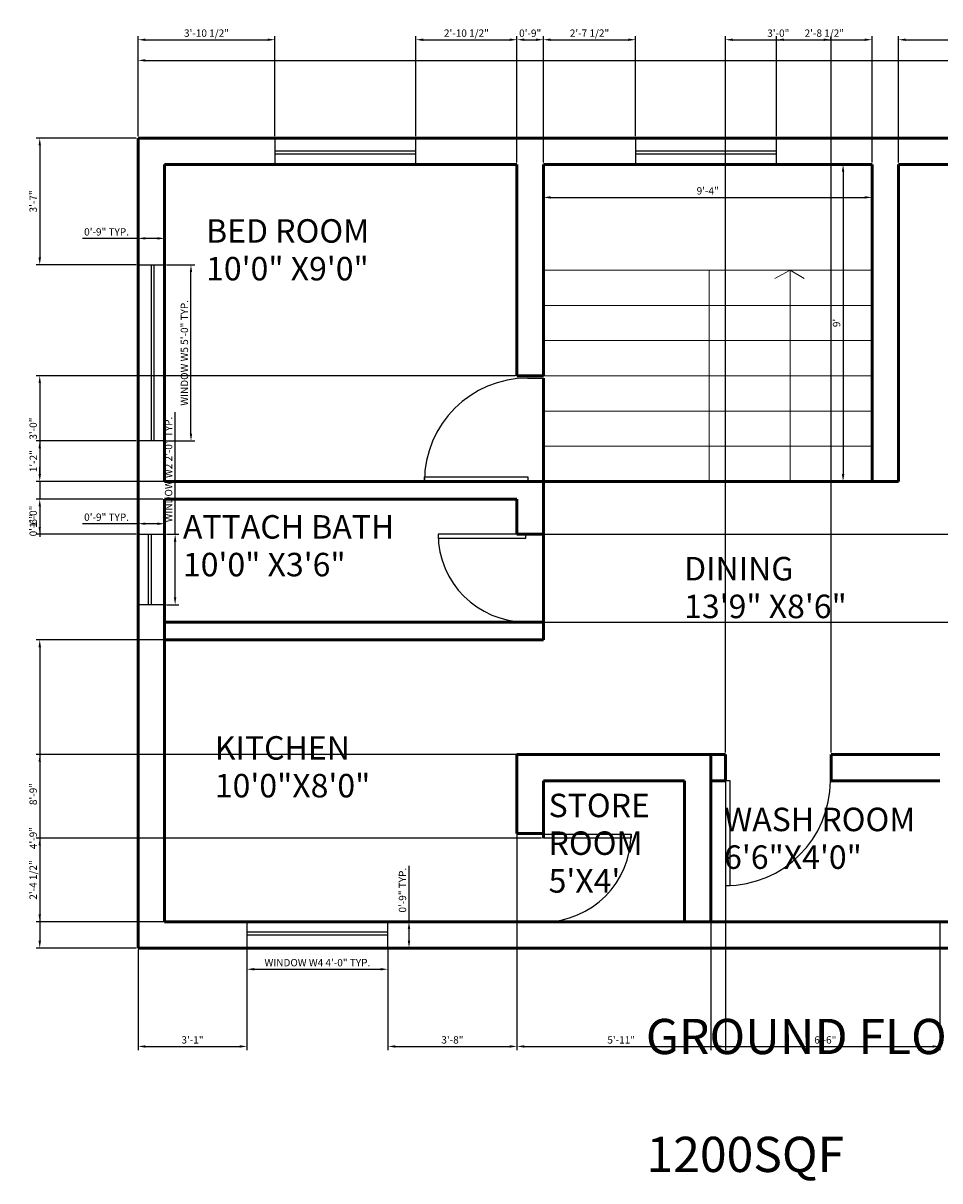
# Model space of a CAD drawing. Units: inches. Extents: x -5798 to 2718, y 1530 to 38999.
# Tile 3 of 4: x 2004 to 2316, y 1947 to 2341. Entities that reach past the tile are written whole.
import ezdxf

# ---------------------------------------------------------------- set-up
doc = ezdxf.new("R2010")
doc.units = ezdxf.units.IN
for name, color, linetype, lineweight in [('A-ANNO-DIMS', 2, 'Continuous', 18), ('A-ANNO-TEXT', 7, 'Continuous', 25), ('A-AREA-IDEN', 3, 'Continuous', 18), ('A-DOOR', 3, 'Continuous', 25), ('A-FLOR-STRS', 8, 'Continuous', 18), ('A-GLAZ', 4, 'Continuous', 25), ('A-WALL', 7, 'Continuous', 50)]:
    doc.layers.add(name, color=color, linetype=linetype, lineweight=lineweight)
doc.styles.get("Standard").update_dxf_attribs({"font": 'arial.ttf'})
doc.dimstyles.new('Copy of ISO-25', dxfattribs={"dimtxt": 2.5, "dimasz": 2.5, "dimexe": 1.25, "dimexo": 0.625, "dimtad": 1, "dimdec": 1, "dimlunit": 4, "dimtxsty": 'Standard', "dimcen": 2.5, "dimadec": 0, "dimazin": 0, "dimtfac": 1, "dimtdec": 1, "dimtmove": 0, "dimatfit": 3, "dimfxl": 1, "dimarcsym": 0})

# ---------------------------------------------------------------- blocks, each defined once
blk = doc.blocks.new('*D4')
at = {"layer": 'A-ANNO-DIMS', "color": 0, "lineweight": -2, "transparency": 16777216}
for p, q in [((2180.98, 2292.65), (2180.98, 2280.8)), ((2292.89, 2292.65), (2292.89, 2280.8)), ((2183.48, 2282.05), (2290.39, 2282.05))]:
    blk.add_line(p, q, dxfattribs=at)
at = {"layer": 'A-ANNO-DIMS', "color": 0, "transparency": 16777216}
for points in [[(2183.48, 2282.47), (2183.48, 2281.64), (2180.98, 2282.05)], [(2290.39, 2282.47), (2290.39, 2281.64), (2292.89, 2282.05)]]:
    blk.add_solid(points, dxfattribs=at)
at = {"layer": 'Defpoints', "color": 0, "transparency": 16777216}
for p in [(2180.98, 2293.28), (2292.89, 2293.28), (2292.89, 2282.05)]:
    blk.add_point(p, dxfattribs=at)
at = {"layer": 'A-ANNO-DIMS', "color": 0, "transparency": 16777216, "insert": (2236.93, 2283.96), "char_height": 2.5, "attachment_point": 5}
blk.add_mtext('9\'-4"', dxfattribs=at)
blk = doc.blocks.new('*U8')
for p, q in [((-40, 0), (-40, 4)), ((0, 0), (0, 4))]:
    blk.add_line(p, q)
blk.add_lwpolyline([(0, 0), (0, -40), (-1.75, -40), (-1.75, 0)], close=True)
blk.add_arc((0, 0), 40, 180, 270)
blk = doc.blocks.new('*U7')
for p, q in [((0, 0), (0, 6)), ((40, 0), (40, 6))]:
    blk.add_line(p, q)
blk.add_lwpolyline([(0, 0), (0, -40), (1.75, -40), (1.75, 0)], close=True)
blk.add_arc((0, 0), 40, 270, 0)
blk = doc.blocks.new('*U5')
for p, q in [((0, 0), (0, -6)), ((-40, 0), (-40, -6))]:
    blk.add_line(p, q)
blk.add_lwpolyline([(0, 0), (0, 40), (-1.75, 40), (-1.75, 0)], close=True)
blk.add_arc((0, 0), 40, 90, 180)
blk = doc.blocks.new('*U2')
for p, q in [((0, 0), (0, -6)), ((40, 0), (40, -6))]:
    blk.add_line(p, q)
blk.add_lwpolyline([(0, 0), (0, 40), (1.75, 40), (1.75, 0)], close=True)
blk.add_arc((0, 0), 40, 0, 90)
blk = doc.blocks.new('*D12')
at = {"layer": 'A-ANNO-DIMS', "color": 0, "lineweight": -2, "transparency": 16777216}
for p, q in [((2292.27, 2293.28), (2281.78, 2293.28)), ((2283.03, 2290.78), (2283.03, 2187.78)), ((2292.27, 2185.28), (2281.78, 2185.28))]:
    blk.add_line(p, q, dxfattribs=at)
at = {"layer": 'A-ANNO-DIMS', "color": 0, "transparency": 16777216}
for points in [[(2282.62, 2290.78), (2283.45, 2290.78), (2283.03, 2293.28)], [(2282.62, 2187.78), (2283.45, 2187.78), (2283.03, 2185.28)]]:
    blk.add_solid(points, dxfattribs=at)
at = {"layer": 'Defpoints', "color": 0, "transparency": 16777216}
for p in [(2292.89, 2293.28), (2283.03, 2185.28), (2292.89, 2185.28)]:
    blk.add_point(p, dxfattribs=at)
at = {"layer": 'A-ANNO-DIMS', "color": 0, "transparency": 16777216, "insert": (2281.13, 2239.28), "char_height": 2.5, "attachment_point": 5, "rotation": 90}
blk.add_mtext("9'", dxfattribs=at)
blk = doc.blocks.new('*D13')
at = {"layer": 'A-ANNO-DIMS', "color": 0, "lineweight": -2, "transparency": 16777216}
for p, q in [((2042.98, 2302.9), (2042.98, 2329.99)), ((2045.48, 2328.74), (2680.39, 2328.74)), ((2682.89, 2302.9), (2682.89, 2329.99))]:
    blk.add_line(p, q, dxfattribs=at)
at = {"layer": 'A-ANNO-DIMS', "color": 0, "transparency": 16777216}
for points in [[(2045.48, 2329.16), (2045.48, 2328.32), (2042.98, 2328.74)], [(2680.39, 2329.16), (2680.39, 2328.32), (2682.89, 2328.74)]]:
    blk.add_solid(points, dxfattribs=at)
at = {"layer": 'Defpoints', "color": 0, "transparency": 16777216}
for p in [(2682.89, 2328.74), (2042.98, 2302.28), (2682.89, 2302.28)]:
    blk.add_point(p, dxfattribs=at)
at = {"layer": 'A-ANNO-DIMS', "color": 0, "transparency": 16777216, "insert": (2362.93, 2330.64), "char_height": 2.5, "attachment_point": 5}
blk.add_mtext('53\'-4"', dxfattribs=at)
blk = doc.blocks.new('WIN-60')
for p, q in [((0, 0), (0, 9)), ((0, 9), (60, 9)), ((60, 9), (60, 0)), ((0, 4.5), (60, 4.5)), ((0, 3.5), (60, 3.5))]:
    blk.add_line(p, q)
blk = doc.blocks.new('WIN-24-B')
for p, q in [((0, 0), (0, 9)), ((0, 9), (24, 9)), ((24, 9), (24, 0)), ((0, 5.5), (24, 5.5)), ((0, 4.5), (24, 4.5))]:
    blk.add_line(p, q)
blk = doc.blocks.new('WIN-48-B')
for p, q in [((0, 9), (0, 0)), ((48, 0), (48, 9)), ((0, 5.5), (48, 5.5)), ((0, 4.5), (48, 4.5)), ((0, 0), (48, 0))]:
    blk.add_line(p, q)
blk = doc.blocks.new('*D24')
at = {"layer": 'A-ANNO-DIMS', "color": 0, "lineweight": -2, "transparency": 16777216}
for p, q in [((2055.58, 2167.28), (2055.58, 2208.87)), ((2052.6, 2167.28), (2056.83, 2167.28)), ((2055.58, 2145.78), (2055.58, 2164.78)), ((2052.6, 2143.28), (2056.83, 2143.28))]:
    blk.add_line(p, q, dxfattribs=at)
at = {"layer": 'A-ANNO-DIMS', "color": 0, "transparency": 16777216}
for points in [[(2055.16, 2164.78), (2055.99, 2164.78), (2055.58, 2167.28)], [(2055.16, 2145.78), (2055.99, 2145.78), (2055.58, 2143.28)]]:
    blk.add_solid(points, dxfattribs=at)
at = {"layer": 'Defpoints', "color": 0, "transparency": 16777216}
for p in [(2051.98, 2167.28), (2055.58, 2167.28), (2051.98, 2143.28)]:
    blk.add_point(p, dxfattribs=at)
at = {"layer": 'A-ANNO-DIMS', "color": 0, "transparency": 16777216, "insert": (2053.66, 2189.33), "char_height": 2.5, "attachment_point": 5, "rotation": 90}
blk.add_mtext('WINDOW W2 2\'-0" TYP.', dxfattribs=at)
blk = doc.blocks.new('*D25')
at = {"layer": 'A-ANNO-DIMS', "color": 0, "lineweight": -2, "transparency": 16777216}
for p, q in [((2042.98, 2170.88), (2023.99, 2170.88)), ((2042.98, 2167.9), (2042.98, 2172.13)), ((2049.48, 2170.88), (2045.48, 2170.88)), ((2051.98, 2167.9), (2051.98, 2172.13))]:
    blk.add_line(p, q, dxfattribs=at)
at = {"layer": 'A-ANNO-DIMS', "color": 0, "transparency": 16777216}
for points in [[(2045.48, 2171.29), (2045.48, 2170.46), (2042.98, 2170.88)], [(2049.48, 2171.29), (2049.48, 2170.46), (2051.98, 2170.88)]]:
    blk.add_solid(points, dxfattribs=at)
at = {"layer": 'Defpoints', "color": 0, "transparency": 16777216}
for p in [(2042.98, 2170.88), (2042.98, 2167.28), (2051.98, 2167.28)]:
    blk.add_point(p, dxfattribs=at)
at = {"layer": 'A-ANNO-DIMS', "color": 0, "transparency": 16777216, "insert": (2032.23, 2172.78), "char_height": 2.5, "attachment_point": 5}
blk.add_mtext('0\'-9" TYP.', dxfattribs=at)
blk = doc.blocks.new('*D28')
at = {"layer": 'A-ANNO-DIMS', "color": 0, "lineweight": -2, "transparency": 16777216}
for p, q in [((2080.02, 2025.65), (2080.02, 2017.83)), ((2128.02, 2025.65), (2128.02, 2017.83)), ((2082.52, 2019.08), (2125.52, 2019.08))]:
    blk.add_line(p, q, dxfattribs=at)
at = {"layer": 'A-ANNO-DIMS', "color": 0, "transparency": 16777216}
for points in [[(2082.52, 2019.49), (2082.52, 2018.66), (2080.02, 2019.08)], [(2125.52, 2019.49), (2125.52, 2018.66), (2128.02, 2019.08)]]:
    blk.add_solid(points, dxfattribs=at)
at = {"layer": 'Defpoints', "color": 0, "transparency": 16777216}
for p in [(2080.02, 2026.28), (2128.02, 2026.28), (2128.02, 2019.08)]:
    blk.add_point(p, dxfattribs=at)
at = {"layer": 'A-ANNO-DIMS', "color": 0, "transparency": 16777216, "insert": (2104.02, 2021), "char_height": 2.5, "attachment_point": 5}
blk.add_mtext('WINDOW W4 4\'-0" TYP.', dxfattribs=at)
blk = doc.blocks.new('*D29')
at = {"layer": 'A-ANNO-DIMS', "color": 0, "lineweight": -2, "transparency": 16777216}
for p, q in [((2135.22, 2035.28), (2135.22, 2054.27)), ((2128.64, 2035.28), (2136.47, 2035.28)), ((2135.22, 2028.78), (2135.22, 2032.78)), ((2128.64, 2026.28), (2136.47, 2026.28))]:
    blk.add_line(p, q, dxfattribs=at)
at = {"layer": 'A-ANNO-DIMS', "color": 0, "transparency": 16777216}
for points in [[(2134.8, 2032.78), (2135.63, 2032.78), (2135.22, 2035.28)], [(2134.8, 2028.78), (2135.63, 2028.78), (2135.22, 2026.28)]]:
    blk.add_solid(points, dxfattribs=at)
at = {"layer": 'Defpoints', "color": 0, "transparency": 16777216}
for p in [(2128.02, 2035.28), (2135.22, 2035.28), (2128.02, 2026.28)]:
    blk.add_point(p, dxfattribs=at)
at = {"layer": 'A-ANNO-DIMS', "color": 0, "transparency": 16777216, "insert": (2133.32, 2046.02), "char_height": 2.5, "attachment_point": 5, "rotation": 90}
blk.add_mtext('0\'-9" TYP.', dxfattribs=at)
blk = doc.blocks.new('*D30')
at = {"layer": 'A-ANNO-DIMS', "color": 0, "lineweight": -2, "transparency": 16777216}
for p, q in [((2052.6, 2259.09), (2062.23, 2259.09)), ((2060.98, 2201.59), (2060.98, 2256.59)), ((2052.6, 2199.09), (2062.23, 2199.09))]:
    blk.add_line(p, q, dxfattribs=at)
at = {"layer": 'A-ANNO-DIMS', "color": 0, "transparency": 16777216}
for points in [[(2060.56, 2256.59), (2061.39, 2256.59), (2060.98, 2259.09)], [(2060.56, 2201.59), (2061.39, 2201.59), (2060.98, 2199.09)]]:
    blk.add_solid(points, dxfattribs=at)
at = {"layer": 'Defpoints', "color": 0, "transparency": 16777216}
for p in [(2051.98, 2259.09), (2060.98, 2259.09), (2051.98, 2199.09)]:
    blk.add_point(p, dxfattribs=at)
at = {"layer": 'A-ANNO-DIMS', "color": 0, "transparency": 16777216, "insert": (2059.06, 2229.09), "char_height": 2.5, "attachment_point": 5, "rotation": 90}
blk.add_mtext('WINDOW W5 5\'-0" TYP.', dxfattribs=at)
blk = doc.blocks.new('*D31')
at = {"layer": 'A-ANNO-DIMS', "color": 0, "lineweight": -2, "transparency": 16777216}
for p, q in [((2042.98, 2268.09), (2023.99, 2268.09)), ((2042.98, 2259.72), (2042.98, 2269.34)), ((2049.48, 2268.09), (2045.48, 2268.09)), ((2051.98, 2259.72), (2051.98, 2269.34))]:
    blk.add_line(p, q, dxfattribs=at)
at = {"layer": 'A-ANNO-DIMS', "color": 0, "transparency": 16777216}
for points in [[(2045.48, 2268.51), (2045.48, 2267.68), (2042.98, 2268.09)], [(2049.48, 2268.51), (2049.48, 2267.68), (2051.98, 2268.09)]]:
    blk.add_solid(points, dxfattribs=at)
at = {"layer": 'Defpoints', "color": 0, "transparency": 16777216}
for p in [(2042.98, 2268.09), (2042.98, 2259.09), (2051.98, 2259.09)]:
    blk.add_point(p, dxfattribs=at)
at = {"layer": 'A-ANNO-DIMS', "color": 0, "transparency": 16777216, "insert": (2032.23, 2269.99), "char_height": 2.5, "attachment_point": 5}
blk.add_mtext('0\'-9" TYP.', dxfattribs=at)
blk = doc.blocks.new('*D32')
at = {"layer": 'A-ANNO-DIMS', "color": 0, "lineweight": -2, "transparency": 16777216}
for p, q in [((2042.98, 2302.9), (2042.98, 2337.03)), ((2045.48, 2335.78), (2087.05, 2335.78)), ((2089.55, 2302.9), (2089.55, 2337.03))]:
    blk.add_line(p, q, dxfattribs=at)
at = {"layer": 'A-ANNO-DIMS', "color": 0, "transparency": 16777216}
for points in [[(2045.48, 2336.19), (2045.48, 2335.36), (2042.98, 2335.78)], [(2087.05, 2336.19), (2087.05, 2335.36), (2089.55, 2335.78)]]:
    blk.add_solid(points, dxfattribs=at)
at = {"layer": 'Defpoints', "color": 0, "transparency": 16777216}
for p in [(2089.55, 2335.78), (2042.98, 2302.28), (2089.55, 2302.28)]:
    blk.add_point(p, dxfattribs=at)
at = {"layer": 'A-ANNO-DIMS', "color": 0, "transparency": 16777216, "insert": (2066.26, 2337.7), "char_height": 2.5, "attachment_point": 5}
blk.add_mtext('3\'-10 1/2"', dxfattribs=at)
blk = doc.blocks.new('*D33')
at = {"layer": 'A-ANNO-DIMS', "color": 0, "lineweight": -2, "transparency": 16777216}
for p, q in [((2137.55, 2302.9), (2137.55, 2337.03)), ((2140.05, 2335.78), (2169.48, 2335.78)), ((2171.98, 2293.9), (2171.98, 2337.03))]:
    blk.add_line(p, q, dxfattribs=at)
at = {"layer": 'A-ANNO-DIMS', "color": 0, "transparency": 16777216}
for points in [[(2140.05, 2336.19), (2140.05, 2335.36), (2137.55, 2335.78)], [(2169.48, 2336.19), (2169.48, 2335.36), (2171.98, 2335.78)]]:
    blk.add_solid(points, dxfattribs=at)
at = {"layer": 'Defpoints', "color": 0, "transparency": 16777216}
for p in [(2171.98, 2335.78), (2137.55, 2302.28), (2171.98, 2293.28)]:
    blk.add_point(p, dxfattribs=at)
at = {"layer": 'A-ANNO-DIMS', "color": 0, "transparency": 16777216, "insert": (2154.76, 2337.7), "char_height": 2.5, "attachment_point": 5}
blk.add_mtext('2\'-10 1/2"', dxfattribs=at)
blk = doc.blocks.new('*D34')
at = {"layer": 'A-ANNO-DIMS', "color": 0, "lineweight": -2, "transparency": 16777216}
for p, q in [((2171.98, 2293.9), (2171.98, 2337.03)), ((2174.48, 2335.78), (2178.48, 2335.78)), ((2180.98, 2293.9), (2180.98, 2337.03))]:
    blk.add_line(p, q, dxfattribs=at)
at = {"layer": 'A-ANNO-DIMS', "color": 0, "transparency": 16777216}
for points in [[(2174.48, 2336.19), (2174.48, 2335.36), (2171.98, 2335.78)], [(2178.48, 2336.19), (2178.48, 2335.36), (2180.98, 2335.78)]]:
    blk.add_solid(points, dxfattribs=at)
at = {"layer": 'Defpoints', "color": 0, "transparency": 16777216}
for p in [(2180.98, 2335.78), (2171.98, 2293.28), (2180.98, 2293.28)]:
    blk.add_point(p, dxfattribs=at)
at = {"layer": 'A-ANNO-DIMS', "color": 0, "transparency": 16777216, "insert": (2176.48, 2337.68), "char_height": 2.5, "attachment_point": 5}
blk.add_mtext('0\'-9"', dxfattribs=at)
blk = doc.blocks.new('*D35')
at = {"layer": 'A-ANNO-DIMS', "color": 0, "lineweight": -2, "transparency": 16777216}
for p, q in [((2180.98, 2293.9), (2180.98, 2337.03)), ((2183.48, 2335.78), (2209.89, 2335.78)), ((2212.39, 2302.9), (2212.39, 2337.03))]:
    blk.add_line(p, q, dxfattribs=at)
at = {"layer": 'A-ANNO-DIMS', "color": 0, "transparency": 16777216}
for points in [[(2183.48, 2336.19), (2183.48, 2335.36), (2180.98, 2335.78)], [(2209.89, 2336.19), (2209.89, 2335.36), (2212.39, 2335.78)]]:
    blk.add_solid(points, dxfattribs=at)
at = {"layer": 'Defpoints', "color": 0, "transparency": 16777216}
for p in [(2212.39, 2335.78), (2212.39, 2302.28), (2180.98, 2293.28)]:
    blk.add_point(p, dxfattribs=at)
at = {"layer": 'A-ANNO-DIMS', "color": 0, "transparency": 16777216, "insert": (2196.68, 2337.7), "char_height": 2.5, "attachment_point": 5}
blk.add_mtext('2\'-7 1/2"', dxfattribs=at)
blk = doc.blocks.new('*D36')
at = {"layer": 'A-ANNO-DIMS', "color": 0, "lineweight": -2, "transparency": 16777216}
for p, q in [((2260.39, 2302.9), (2260.39, 2337.03)), ((2262.89, 2335.78), (2290.39, 2335.78)), ((2292.89, 2293.9), (2292.89, 2337.03))]:
    blk.add_line(p, q, dxfattribs=at)
at = {"layer": 'A-ANNO-DIMS', "color": 0, "transparency": 16777216}
for points in [[(2262.89, 2336.19), (2262.89, 2335.36), (2260.39, 2335.78)], [(2290.39, 2336.19), (2290.39, 2335.36), (2292.89, 2335.78)]]:
    blk.add_solid(points, dxfattribs=at)
at = {"layer": 'Defpoints', "color": 0, "transparency": 16777216}
for p in [(2292.89, 2335.78), (2260.39, 2302.28), (2292.89, 2293.28)]:
    blk.add_point(p, dxfattribs=at)
at = {"layer": 'A-ANNO-DIMS', "color": 0, "transparency": 16777216, "insert": (2276.64, 2337.7), "char_height": 2.5, "attachment_point": 5}
blk.add_mtext('2\'-8 1/2"', dxfattribs=at)
blk = doc.blocks.new('*D37')
at = {"layer": 'A-ANNO-DIMS', "color": 0, "lineweight": -2, "transparency": 16777216}
for p, q in [((2301.89, 2293.9), (2301.89, 2337.03)), ((2304.39, 2335.78), (2341.39, 2335.78)), ((2343.89, 2293.9), (2343.89, 2337.03))]:
    blk.add_line(p, q, dxfattribs=at)
at = {"layer": 'A-ANNO-DIMS', "color": 0, "transparency": 16777216}
for points in [[(2304.39, 2336.19), (2304.39, 2335.36), (2301.89, 2335.78)], [(2341.39, 2336.19), (2341.39, 2335.36), (2343.89, 2335.78)]]:
    blk.add_solid(points, dxfattribs=at)
at = {"layer": 'Defpoints', "color": 0, "transparency": 16777216}
for p in [(2343.89, 2335.78), (2301.89, 2293.28), (2343.89, 2293.28)]:
    blk.add_point(p, dxfattribs=at)
at = {"layer": 'A-ANNO-DIMS', "color": 0, "transparency": 16777216, "insert": (2322.89, 2337.68), "char_height": 2.5, "attachment_point": 5}
blk.add_mtext('3\'-6"', dxfattribs=at)
blk = doc.blocks.new('*D39')
at = {"layer": 'A-ANNO-DIMS', "color": 0, "lineweight": -2, "transparency": 16777216}
for p, q in [((2042.35, 2302.28), (2008.23, 2302.28)), ((2009.48, 2299.78), (2009.48, 2261.59)), ((2042.35, 2259.09), (2008.23, 2259.09))]:
    blk.add_line(p, q, dxfattribs=at)
at = {"layer": 'A-ANNO-DIMS', "color": 0, "transparency": 16777216}
for points in [[(2009.06, 2299.78), (2009.89, 2299.78), (2009.48, 2302.28)], [(2009.06, 2261.59), (2009.89, 2261.59), (2009.48, 2259.09)]]:
    blk.add_solid(points, dxfattribs=at)
at = {"layer": 'Defpoints', "color": 0, "transparency": 16777216}
for p in [(2042.98, 2302.28), (2009.48, 2259.09), (2042.98, 2259.09)]:
    blk.add_point(p, dxfattribs=at)
at = {"layer": 'A-ANNO-DIMS', "color": 0, "transparency": 16777216, "insert": (2007.57, 2280.69), "char_height": 2.5, "attachment_point": 5, "rotation": 90}
blk.add_mtext('3\'-7"', dxfattribs=at)
blk = doc.blocks.new('*D40')
at = {"layer": 'A-ANNO-DIMS', "color": 0, "lineweight": -2, "transparency": 16777216}
for p, q in [((2042.35, 2199.09), (2008.23, 2199.09)), ((2009.48, 2196.59), (2009.48, 2187.78)), ((2051.35, 2185.28), (2008.23, 2185.28))]:
    blk.add_line(p, q, dxfattribs=at)
at = {"layer": 'A-ANNO-DIMS', "color": 0, "transparency": 16777216}
for points in [[(2009.06, 2196.59), (2009.89, 2196.59), (2009.48, 2199.09)], [(2009.06, 2187.78), (2009.89, 2187.78), (2009.48, 2185.28)]]:
    blk.add_solid(points, dxfattribs=at)
at = {"layer": 'Defpoints', "color": 0, "transparency": 16777216}
for p in [(2042.98, 2199.09), (2009.48, 2185.28), (2051.98, 2185.28)]:
    blk.add_point(p, dxfattribs=at)
at = {"layer": 'A-ANNO-DIMS', "color": 0, "transparency": 16777216, "insert": (2007.6, 2192.19), "char_height": 2.5, "attachment_point": 5, "rotation": 90}
blk.add_mtext('1\'-2"', dxfattribs=at)
blk = doc.blocks.new('*D41')
at = {"layer": 'A-ANNO-DIMS', "color": 0, "lineweight": -2, "transparency": 16777216}
for p, q in [((2009.48, 2187.78), (2009.48, 2190.28)), ((2051.35, 2185.28), (2008.23, 2185.28)), ((2009.48, 2185.28), (2009.48, 2179.28)), ((2051.35, 2179.28), (2008.23, 2179.28)), ((2009.48, 2176.78), (2009.48, 2166.38))]:
    blk.add_line(p, q, dxfattribs=at)
at = {"layer": 'A-ANNO-DIMS', "color": 0, "transparency": 16777216}
for points in [[(2009.06, 2187.78), (2009.89, 2187.78), (2009.48, 2185.28)], [(2009.06, 2176.78), (2009.89, 2176.78), (2009.48, 2179.28)]]:
    blk.add_solid(points, dxfattribs=at)
at = {"layer": 'Defpoints', "color": 0, "transparency": 16777216}
for p in [(2051.98, 2185.28), (2009.48, 2179.28), (2051.98, 2179.28)]:
    blk.add_point(p, dxfattribs=at)
at = {"layer": 'A-ANNO-DIMS', "color": 0, "transparency": 16777216, "insert": (2007.57, 2170.33), "char_height": 2.5, "attachment_point": 5, "rotation": 90}
blk.add_mtext('0\'-6"', dxfattribs=at)
blk = doc.blocks.new('*D42')
at = {"layer": 'A-ANNO-DIMS', "color": 0, "lineweight": -2, "transparency": 16777216}
for p, q in [((2051.35, 2179.28), (2008.23, 2179.28)), ((2009.48, 2176.78), (2009.48, 2169.78)), ((2042.35, 2167.28), (2008.23, 2167.28))]:
    blk.add_line(p, q, dxfattribs=at)
at = {"layer": 'A-ANNO-DIMS', "color": 0, "transparency": 16777216}
for points in [[(2009.06, 2176.78), (2009.89, 2176.78), (2009.48, 2179.28)], [(2009.06, 2169.78), (2009.89, 2169.78), (2009.48, 2167.28)]]:
    blk.add_solid(points, dxfattribs=at)
at = {"layer": 'Defpoints', "color": 0, "transparency": 16777216}
for p in [(2051.98, 2179.28), (2009.48, 2167.28), (2042.98, 2167.28)]:
    blk.add_point(p, dxfattribs=at)
at = {"layer": 'A-ANNO-DIMS', "color": 0, "transparency": 16777216, "insert": (2007.57, 2173.28), "char_height": 2.5, "attachment_point": 5, "rotation": 90}
blk.add_mtext('1\'-0"', dxfattribs=at)
blk = doc.blocks.new('*D43')
at = {"layer": 'A-ANNO-DIMS', "color": 0, "lineweight": -2, "transparency": 16777216}
for p, q in [((2051.35, 2131.28), (2008.23, 2131.28)), ((2009.48, 2128.78), (2009.48, 2028.78)), ((2042.35, 2026.28), (2008.23, 2026.28))]:
    blk.add_line(p, q, dxfattribs=at)
at = {"layer": 'A-ANNO-DIMS', "color": 0, "transparency": 16777216}
for points in [[(2009.06, 2128.78), (2009.89, 2128.78), (2009.48, 2131.28)], [(2009.06, 2028.78), (2009.89, 2028.78), (2009.48, 2026.28)]]:
    blk.add_solid(points, dxfattribs=at)
at = {"layer": 'Defpoints', "color": 0, "transparency": 16777216}
for p in [(2051.98, 2131.28), (2009.48, 2026.28), (2042.98, 2026.28)]:
    blk.add_point(p, dxfattribs=at)
at = {"layer": 'A-ANNO-DIMS', "color": 0, "transparency": 16777216, "insert": (2007.57, 2078.78), "char_height": 2.5, "attachment_point": 5, "rotation": 90}
blk.add_mtext('8\'-9"', dxfattribs=at)
blk = doc.blocks.new('*D47')
at = {"layer": 'A-ANNO-DIMS', "color": 0, "lineweight": -2, "transparency": 16777216}
for p, q in [((2042.98, 2025.65), (2042.98, 1991.53)), ((2080.02, 2025.65), (2080.02, 1991.53)), ((2045.48, 1992.78), (2077.52, 1992.78))]:
    blk.add_line(p, q, dxfattribs=at)
at = {"layer": 'A-ANNO-DIMS', "color": 0, "transparency": 16777216}
for points in [[(2045.48, 1993.19), (2045.48, 1992.36), (2042.98, 1992.78)], [(2077.52, 1993.19), (2077.52, 1992.36), (2080.02, 1992.78)]]:
    blk.add_solid(points, dxfattribs=at)
at = {"layer": 'Defpoints', "color": 0, "transparency": 16777216}
for p in [(2042.98, 2026.28), (2080.02, 2026.28), (2080.02, 1992.78)]:
    blk.add_point(p, dxfattribs=at)
at = {"layer": 'A-ANNO-DIMS', "color": 0, "transparency": 16777216, "insert": (2061.5, 1994.68), "char_height": 2.5, "attachment_point": 5}
blk.add_mtext('3\'-1"', dxfattribs=at)
blk = doc.blocks.new('*D48')
at = {"layer": 'A-ANNO-DIMS', "color": 0, "lineweight": -2, "transparency": 16777216}
for p, q in [((2171.98, 2091.65), (2171.98, 1991.53)), ((2128.02, 2025.65), (2128.02, 1991.53)), ((2130.52, 1992.78), (2169.48, 1992.78))]:
    blk.add_line(p, q, dxfattribs=at)
at = {"layer": 'A-ANNO-DIMS', "color": 0, "transparency": 16777216}
for points in [[(2130.52, 1993.19), (2130.52, 1992.36), (2128.02, 1992.78)], [(2169.48, 1993.19), (2169.48, 1992.36), (2171.98, 1992.78)]]:
    blk.add_solid(points, dxfattribs=at)
at = {"layer": 'Defpoints', "color": 0, "transparency": 16777216}
for p in [(2171.98, 2092.28), (2128.02, 2026.28), (2171.98, 1992.78)]:
    blk.add_point(p, dxfattribs=at)
at = {"layer": 'A-ANNO-DIMS', "color": 0, "transparency": 16777216, "insert": (2150, 1994.68), "char_height": 2.5, "attachment_point": 5}
blk.add_mtext('3\'-8"', dxfattribs=at)
blk = doc.blocks.new('*D49')
at = {"layer": 'A-ANNO-DIMS', "color": 0, "lineweight": -2, "transparency": 16777216}
for p, q in [((2237.98, 2034.65), (2237.98, 1991.53)), ((2315.98, 2034.65), (2315.98, 1991.53)), ((2240.48, 1992.78), (2313.48, 1992.78))]:
    blk.add_line(p, q, dxfattribs=at)
at = {"layer": 'A-ANNO-DIMS', "color": 0, "transparency": 16777216}
for points in [[(2240.48, 1993.19), (2240.48, 1992.36), (2237.98, 1992.78)], [(2313.48, 1993.19), (2313.48, 1992.36), (2315.98, 1992.78)]]:
    blk.add_solid(points, dxfattribs=at)
at = {"layer": 'Defpoints', "color": 0, "transparency": 16777216}
for p in [(2237.98, 2035.28), (2315.98, 2035.28), (2315.98, 1992.78)]:
    blk.add_point(p, dxfattribs=at)
at = {"layer": 'A-ANNO-DIMS', "color": 0, "transparency": 16777216, "insert": (2276.98, 1994.68), "char_height": 2.5, "attachment_point": 5}
blk.add_mtext('6\'-6"', dxfattribs=at)
blk = doc.blocks.new('*D53')
at = {"layer": 'A-ANNO-DIMS', "color": 0, "lineweight": -2, "transparency": 16777216}
for p, q in [((2171.98, 2091.65), (2171.98, 1991.53)), ((2242.97, 2091.65), (2242.97, 1991.53)), ((2174.48, 1992.78), (2240.47, 1992.78))]:
    blk.add_line(p, q, dxfattribs=at)
at = {"layer": 'A-ANNO-DIMS', "color": 0, "transparency": 16777216}
for points in [[(2174.48, 1993.19), (2174.48, 1992.36), (2171.98, 1992.78)], [(2240.47, 1993.19), (2240.47, 1992.36), (2242.97, 1992.78)]]:
    blk.add_solid(points, dxfattribs=at)
at = {"layer": 'Defpoints', "color": 0, "transparency": 16777216}
for p in [(2171.98, 2092.28), (2242.97, 2092.28), (2242.97, 1992.78)]:
    blk.add_point(p, dxfattribs=at)
at = {"layer": 'A-ANNO-DIMS', "color": 0, "transparency": 16777216, "insert": (2207.47, 1994.68), "char_height": 2.5, "attachment_point": 5}
blk.add_mtext('5\'-11"', dxfattribs=at)
blk = doc.blocks.new('*D54')
at = {"layer": 'A-ANNO-DIMS', "color": 0, "lineweight": -2, "transparency": 16777216}
for p, q in [((2242.34, 2092.28), (2008.23, 2092.28)), ((2009.48, 2089.78), (2009.48, 2037.78)), ((2237.35, 2035.28), (2008.23, 2035.28))]:
    blk.add_line(p, q, dxfattribs=at)
at = {"layer": 'A-ANNO-DIMS', "color": 0, "transparency": 16777216}
for points in [[(2009.06, 2089.78), (2009.89, 2089.78), (2009.48, 2092.28)], [(2009.06, 2037.78), (2009.89, 2037.78), (2009.48, 2035.28)]]:
    blk.add_solid(points, dxfattribs=at)
at = {"layer": 'Defpoints', "color": 0, "transparency": 16777216}
for p in [(2242.97, 2092.28), (2009.48, 2035.28), (2237.98, 2035.28)]:
    blk.add_point(p, dxfattribs=at)
at = {"layer": 'A-ANNO-DIMS', "color": 0, "transparency": 16777216, "insert": (2007.57, 2063.78), "char_height": 2.5, "attachment_point": 5, "rotation": 90}
blk.add_mtext('4\'-9"', dxfattribs=at)
blk = doc.blocks.new('*D58')
at = {"layer": 'A-ANNO-DIMS', "color": 0, "lineweight": -2, "transparency": 16777216}
for p, q in [((2171.35, 2221.28), (2008.23, 2221.28)), ((2009.48, 2218.78), (2009.48, 2187.78)), ((2171.35, 2185.28), (2008.23, 2185.28))]:
    blk.add_line(p, q, dxfattribs=at)
at = {"layer": 'A-ANNO-DIMS', "color": 0, "transparency": 16777216}
for points in [[(2009.06, 2218.78), (2009.89, 2218.78), (2009.48, 2221.28)], [(2009.06, 2187.78), (2009.89, 2187.78), (2009.48, 2185.28)]]:
    blk.add_solid(points, dxfattribs=at)
at = {"layer": 'Defpoints', "color": 0, "transparency": 16777216}
for p in [(2171.98, 2221.28), (2009.48, 2185.28), (2171.98, 2185.28)]:
    blk.add_point(p, dxfattribs=at)
at = {"layer": 'A-ANNO-DIMS', "color": 0, "transparency": 16777216, "insert": (2007.57, 2203.28), "char_height": 2.5, "attachment_point": 5, "rotation": 90}
blk.add_mtext('3\'-0"', dxfattribs=at)
blk = doc.blocks.new('*D59')
at = {"layer": 'A-ANNO-DIMS', "color": 0, "lineweight": -2, "transparency": 16777216}
for p, q in [((2181.6, 2167.28), (2717.64, 2167.28)), ((2716.39, 2164.78), (2716.39, 2139.78)), ((2181.6, 2137.28), (2717.64, 2137.28))]:
    blk.add_line(p, q, dxfattribs=at)
at = {"layer": 'A-ANNO-DIMS', "color": 0, "transparency": 16777216}
for points in [[(2715.98, 2164.78), (2716.81, 2164.78), (2716.39, 2167.28)], [(2715.98, 2139.78), (2716.81, 2139.78), (2716.39, 2137.28)]]:
    blk.add_solid(points, dxfattribs=at)
at = {"layer": 'Defpoints', "color": 0, "transparency": 16777216}
for p in [(2180.98, 2167.28), (2180.98, 2137.28), (2716.39, 2137.28)]:
    blk.add_point(p, dxfattribs=at)
at = {"layer": 'A-ANNO-DIMS', "color": 0, "transparency": 16777216, "insert": (2714.49, 2152.28), "char_height": 2.5, "attachment_point": 5, "rotation": 90}
blk.add_mtext('2\'-6"', dxfattribs=at)
blk = doc.blocks.new('*D60')
at = {"layer": 'A-ANNO-DIMS', "color": 0, "lineweight": -2, "transparency": 16777216}
for p, q in [((2180.35, 2063.78), (2008.23, 2063.78)), ((2009.48, 2061.28), (2009.48, 2037.72)), ((2177.36, 2035.22), (2008.23, 2035.22))]:
    blk.add_line(p, q, dxfattribs=at)
at = {"layer": 'A-ANNO-DIMS', "color": 0, "transparency": 16777216}
for points in [[(2009.06, 2061.28), (2009.89, 2061.28), (2009.48, 2063.78)], [(2009.06, 2037.72), (2009.89, 2037.72), (2009.48, 2035.22)]]:
    blk.add_solid(points, dxfattribs=at)
at = {"layer": 'Defpoints', "color": 0, "transparency": 16777216}
for p in [(2180.98, 2063.78), (2009.48, 2035.22), (2177.99, 2035.22)]:
    blk.add_point(p, dxfattribs=at)
at = {"layer": 'A-ANNO-DIMS', "color": 0, "transparency": 16777216, "insert": (2007.56, 2049.5), "char_height": 2.5, "attachment_point": 5, "rotation": 90}
blk.add_mtext('2\'-4 1/2"', dxfattribs=at)
blk = doc.blocks.new('*D61')
at = {"layer": 'A-ANNO-DIMS', "color": 0, "lineweight": -2, "transparency": 16777216}
for p, q in [((2242.97, 2092.9), (2242.97, 2337.03)), ((2245.47, 2335.78), (2276.47, 2335.78)), ((2278.97, 2092.9), (2278.97, 2337.03))]:
    blk.add_line(p, q, dxfattribs=at)
at = {"layer": 'A-ANNO-DIMS', "color": 0, "transparency": 16777216}
for points in [[(2245.47, 2336.19), (2245.47, 2335.36), (2242.97, 2335.78)], [(2276.47, 2336.19), (2276.47, 2335.36), (2278.97, 2335.78)]]:
    blk.add_solid(points, dxfattribs=at)
at = {"layer": 'Defpoints', "color": 0, "transparency": 16777216}
for p in [(2278.97, 2335.78), (2242.97, 2092.28), (2278.97, 2092.28)]:
    blk.add_point(p, dxfattribs=at)
at = {"layer": 'A-ANNO-DIMS', "color": 0, "transparency": 16777216, "insert": (2260.97, 2337.68), "char_height": 2.5, "attachment_point": 5}
blk.add_mtext('3\'-0"', dxfattribs=at)

msp = doc.modelspace()

# ---------------------------------------------------------------- linework, layer by layer
at = {"layer": 'A-FLOR-STRS'}
for p, q in [((2180.98, 2257.28), (2292.89, 2257.28)), ((2237.38, 2185.28), (2237.38, 2257.28)), ((2265.03, 2257.28), (2259.83, 2254.46)), ((2265.03, 2185.28), (2265.03, 2257.28)), ((2265.03, 2257.28), (2269.76, 2254.46)), ((2180.98, 2245.28), (2292.89, 2245.28)), ((2180.98, 2233.28), (2292.89, 2233.28)), ((2180.98, 2221.28), (2292.89, 2221.28)), ((2180.98, 2209.28), (2292.89, 2209.28)), ((2180.98, 2197.28), (2292.89, 2197.28))]:
    msp.add_line(p, q, dxfattribs=at)
at = {"layer": 'A-WALL'}
for p, q in [((2042.98, 2302.28), (2051.98, 2302.28)), ((2042.98, 2302.28), (2042.98, 2293.28)), ((2051.98, 2302.28), (2171.98, 2302.28)), ((2171.98, 2302.28), (2180.98, 2302.28)), ((2180.98, 2302.28), (2292.89, 2302.28)), ((2292.89, 2302.28), (2301.89, 2302.28)), ((2301.89, 2302.28), (2541.89, 2302.28)), ((2042.98, 2293.28), (2042.98, 2185.28)), ((2051.98, 2194.28), (2051.98, 2293.28)), ((2051.98, 2293.28), (2171.98, 2293.28)), ((2051.98, 2293.28), (2051.98, 2185.28)), ((2051.98, 2293.28), (2051.98, 2259.09)), ((2171.98, 2221.28), (2171.98, 2293.28)), ((2180.98, 2293.28), (2180.98, 2221.28)), ((2292.89, 2293.28), (2180.98, 2293.28)), ((2292.89, 2293.28), (2292.89, 2185.28)), ((2301.89, 2185.28), (2301.89, 2293.28)), ((2343.89, 2293.28), (2301.89, 2293.28)), ((2180.98, 2221.28), (2171.98, 2221.28)), ((2180.98, 2220.51), (2180.98, 2185.28)), ((2051.98, 2194.28), (2051.98, 2185.28)), ((2042.98, 2026.28), (2042.98, 2185.28)), ((2051.98, 2185.28), (2171.98, 2185.28)), ((2171.98, 2185.28), (2180.98, 2185.28)), ((2180.98, 2143.28), (2180.98, 2185.28)), ((2180.98, 2185.28), (2292.89, 2185.28)), ((2180.98, 2185.28), (2237.38, 2185.28)), ((2292.89, 2185.28), (2301.89, 2185.28)), ((2051.98, 2179.28), (2051.98, 2035.28)), ((2051.98, 2179.28), (2051.98, 2143.28)), ((2171.98, 2179.28), (2051.98, 2179.28)), ((2051.98, 2179.28), (2051.98, 2167.28)), ((2171.98, 2179.28), (2171.98, 2167.28)), ((2171.98, 2179.28), (2171.98, 2167.28)), ((2180.98, 2167.28), (2171.98, 2167.28)), ((2180.98, 2137.28), (2180.98, 2167.28)), ((2180.98, 2143.28), (2180.98, 2137.28)), ((2171.98, 2137.28), (2051.98, 2137.28)), ((2171.98, 2137.28), (2180.98, 2137.28)), ((2180.98, 2137.28), (2180.98, 2131.28)), ((2180.98, 2131.28), (2051.98, 2131.28)), ((2051.98, 2131.28), (2051.98, 2035.28)), ((2171.98, 2083.28), (2171.98, 2092.28)), ((2171.98, 2092.28), (2180.98, 2092.28)), ((2180.98, 2092.28), (2228.98, 2092.28)), ((2228.98, 2092.28), (2237.98, 2092.28)), ((2237.98, 2092.28), (2242.97, 2092.28)), ((2237.98, 2083.28), (2237.98, 2092.28)), ((2242.97, 2083.28), (2242.97, 2092.28)), ((2278.97, 2083.28), (2278.97, 2092.28)), ((2278.97, 2092.28), (2315.98, 2092.28)), ((2171.98, 2073.84), (2171.98, 2083.28)), ((2180.98, 2073.84), (2180.98, 2083.28)), ((2228.98, 2083.28), (2180.98, 2083.28)), ((2180.98, 2083.28), (2180.98, 2073.84)), ((2228.98, 2035.28), (2228.98, 2083.28)), ((2237.98, 2083.28), (2237.98, 2035.28)), ((2237.98, 2083.28), (2242.97, 2083.28)), ((2237.98, 2083.28), (2242.97, 2083.28)), ((2278.97, 2083.28), (2315.98, 2083.28)), ((2171.98, 2073.84), (2171.98, 2065.28)), ((2180.98, 2073.84), (2180.98, 2063.78)), ((2180.98, 2065.28), (2171.98, 2065.28)), ((2180.98, 2063.78), (2180.98, 2065.28)), ((2051.98, 2035.28), (2571.89, 2035.28)), ((2051.98, 2035.28), (2171.98, 2035.28)), ((2171.98, 2035.28), (2180.98, 2035.28)), ((2237.98, 2035.28), (2228.98, 2035.28)), ((2682.89, 2026.28), (2042.98, 2026.28))]:
    msp.add_line(p, q, dxfattribs=at)

# ---------------------------------------------------------------- block references
at = {"layer": 'A-DOOR', "rotation": 90}
for name, p, xscale, yscale, zscale in [('*U2', (2175.69, 2185.28), 0.8808171385769682, 0.8808171385769682, 0.8808171385769682), ('*U5', (2175, 2167.28), 0.746256712766472, 0.746256712766472, 0.746256712766472), ('*U8', (2180.98, 2065.09), 0.7465747895484535, 0.7465747895484535, 0.7465747895484535)]:
    msp.add_blockref(name, p, dxfattribs=dict(at, xscale=xscale, yscale=yscale, zscale=zscale))
at = {"layer": 'A-DOOR', "xscale": 0.8930318424856681, "yscale": 0.8930318424856681, "zscale": 0.8930318424856681}
msp.add_blockref('*U7', (2242.97, 2083.28), dxfattribs=at)
at = {"layer": 'A-GLAZ'}
for name, p, rotation in [('WIN-48-B', (2137.55, 2302.28), 180), ('WIN-48-B', (2260.39, 2302.28), 180), ('WIN-60', (2051.98, 2199.09), 90.00000000000014), ('WIN-24-B', (2051.98, 2143.28), 89.9999999999991)]:
    msp.add_blockref(name, p, dxfattribs=dict(at, rotation=rotation))
msp.add_blockref('WIN-48-B', (2080.02, 2026.28), dxfattribs=at)

# ---------------------------------------------------------------- texts
at = {"layer": 'A-ANNO-TEXT'}
for s, p in [('GROUND FLOOR ', (2215.86, 1990.17)), ('1200SQF', (2216.11, 1950))]:
    msp.add_text(s, height=12, dxfattribs=at).set_placement(p)
at = {"layer": 'A-AREA-IDEN'}
for s, p in [('BED ROOM ', (2066.11, 2266.63)), ('10\'0" X9\'0"', (2066.11, 2253.78)), ('ATTACH BATH', (2058.23, 2165.8)), ('10\'0" X3\'6"', (2058.23, 2152.95)), ('DINING', (2228.89, 2151.55)), ('13\'9" X8\'6"', (2228.89, 2138.7)), ('KITCHEN', (2069.09, 2090.49)), ('10\'0"X8\'0"', (2069.09, 2077.63)), ('STORE', (2182.75, 2070.89)), ('WASH ROOM', (2242.52, 2066.12)), ('ROOM', (2182.75, 2058.04)), ('6\'6"X4\'0"', (2242.52, 2053.27)), ("5'X4'", (2182.75, 2045.19))]:
    msp.add_text(s, height=8, dxfattribs=at).set_placement(p)

# ---------------------------------------------------------------- dimensions: what is measured, and where the dimension line sits
at = {"layer": 'A-ANNO-DIMS'}
for base, p1, p2, override, picture, middle in [((2089.55, 2335.78), (2042.98, 2302.28), (2089.55, 2302.28), {"dimdec": 1, "dimlfac": 1, "dimrnd": 0, "dimzin": 1, "dimdsep": 46, "dimlunit": 4, "dimfrac": 2}, '*D32', (2066.26, 2337.7)), ((2171.98, 2335.78), (2137.55, 2302.28), (2171.98, 2293.28), {"dimdec": 1, "dimlfac": 1, "dimrnd": 0, "dimzin": 1, "dimdsep": 46, "dimlunit": 4, "dimfrac": 2}, '*D33', (2154.76, 2337.7)), ((2180.98, 2335.78), (2171.98, 2293.28), (2180.98, 2293.28), {"dimdec": 1, "dimlfac": 1, "dimrnd": 0, "dimzin": 1, "dimdsep": 46, "dimlunit": 4, "dimfrac": 2}, '*D34', (2176.48, 2337.68)), ((2212.39, 2335.78), (2180.98, 2293.28), (2212.39, 2302.28), {"dimdec": 1, "dimlfac": 1, "dimrnd": 0, "dimzin": 1, "dimdsep": 46, "dimlunit": 4, "dimfrac": 2}, '*D35', (2196.68, 2337.7)), ((2278.97, 2335.78), (2242.97, 2092.28), (2278.97, 2092.28), {"dimdec": 1, "dimlfac": 1, "dimrnd": 0, "dimzin": 1, "dimdsep": 46, "dimlunit": 4, "dimfrac": 2}, '*D61', (2260.97, 2337.68)), ((2292.89, 2335.78), (2260.39, 2302.28), (2292.89, 2293.28), {"dimdec": 1, "dimlfac": 1, "dimrnd": 0, "dimzin": 1, "dimdsep": 46, "dimlunit": 4, "dimfrac": 2}, '*D36', (2276.64, 2337.7)), ((2343.89, 2335.78), (2301.89, 2293.28), (2343.89, 2293.28), {"dimdec": 1, "dimlfac": 1, "dimrnd": 0, "dimzin": 1, "dimdsep": 46, "dimlunit": 4, "dimfrac": 2}, '*D37', (2322.89, 2337.68)), ((2682.89, 2328.74), (2042.98, 2302.28), (2682.89, 2302.28), {"dimclrd": 0, "dimclre": 0, "dimclrt": 0}, '*D13', (2362.93, 2330.64)), ((2292.89, 2282.05), (2180.98, 2293.28), (2292.89, 2293.28), {"dimclrd": 0, "dimclre": 0, "dimclrt": 0}, '*D4', (2236.93, 2283.96)), ((2171.98, 1992.78), (2128.02, 2026.28), (2171.98, 2092.28), {"dimdec": 1, "dimlfac": 1, "dimrnd": 0, "dimzin": 1, "dimdsep": 46, "dimlunit": 4, "dimfrac": 2}, '*D48', (2150, 1994.68)), ((2242.97, 1992.78), (2171.98, 2092.28), (2242.97, 2092.28), {"dimdec": 1, "dimlfac": 1, "dimrnd": 0, "dimzin": 1, "dimdsep": 46, "dimlunit": 4, "dimfrac": 2}, '*D53', (2207.47, 1994.68)), ((2315.98, 1992.78), (2237.98, 2035.28), (2315.98, 2035.28), {"dimdec": 1, "dimlfac": 1, "dimrnd": 0, "dimzin": 1, "dimdsep": 46, "dimlunit": 4, "dimfrac": 2}, '*D49', (2276.98, 1994.68)), ((2080.02, 1992.78), (2042.98, 2026.28), (2080.02, 2026.28), {"dimdec": 1, "dimlfac": 1, "dimrnd": 0, "dimzin": 1, "dimdsep": 46, "dimlunit": 4, "dimfrac": 2}, '*D47', (2061.5, 1994.68))]:
    dim = msp.add_linear_dim(base=base, p1=p1, p2=p2, dimstyle='Copy of ISO-25', override=override, dxfattribs=at)
    dim.commit()
    dim.dimension.update_dxf_attribs({"geometry": picture, "text_midpoint": middle})
for base, p1, p2, override, picture, middle in [((2009.48, 2259.09), (2042.98, 2302.28), (2042.98, 2259.09), {"dimdec": 1, "dimlfac": 1, "dimrnd": 0, "dimzin": 1, "dimdsep": 46, "dimlunit": 4, "dimfrac": 2}, '*D39', (2007.57, 2280.69)), ((2283.03, 2185.28), (2292.89, 2293.28), (2292.89, 2185.28), {"dimclrd": 0, "dimclre": 0, "dimclrt": 0}, '*D12', (2281.13, 2239.28)), ((2009.48, 2185.28), (2171.98, 2221.28), (2171.98, 2185.28), {"dimdec": 1, "dimlfac": 1, "dimrnd": 0, "dimzin": 1, "dimdsep": 46, "dimlunit": 4, "dimfrac": 2}, '*D58', (2007.57, 2203.28)), ((2009.48, 2185.28), (2042.98, 2199.09), (2051.98, 2185.28), {"dimdec": 1, "dimlfac": 1, "dimrnd": 0, "dimzin": 1, "dimdsep": 46, "dimlunit": 4, "dimfrac": 2}, '*D40', (2007.6, 2192.19)), ((2009.48, 2179.28), (2051.98, 2185.28), (2051.98, 2179.28), {"dimdec": 1, "dimlfac": 1, "dimrnd": 0, "dimzin": 1, "dimdsep": 46, "dimlunit": 4, "dimfrac": 2}, '*D41', (2007.57, 2170.33)), ((2009.48, 2167.28), (2051.98, 2179.28), (2042.98, 2167.28), {"dimdec": 1, "dimlfac": 1, "dimrnd": 0, "dimzin": 1, "dimdsep": 46, "dimlunit": 4, "dimfrac": 2}, '*D42', (2007.57, 2173.28)), ((2716.39, 2137.28), (2180.98, 2167.28), (2180.98, 2137.28), {"dimdec": 1, "dimlfac": 1, "dimrnd": 0, "dimzin": 1, "dimdsep": 46, "dimlunit": 4, "dimfrac": 2}, '*D59', (2714.49, 2152.28)), ((2009.48, 2026.28), (2051.98, 2131.28), (2042.98, 2026.28), {"dimdec": 1, "dimlfac": 1, "dimrnd": 0, "dimzin": 1, "dimdsep": 46, "dimlunit": 4, "dimfrac": 2}, '*D43', (2007.57, 2078.78)), ((2009.48, 2035.28), (2242.97, 2092.28), (2237.98, 2035.28), {"dimdec": 1, "dimlfac": 1, "dimrnd": 0, "dimzin": 1, "dimdsep": 46, "dimlunit": 4, "dimfrac": 2}, '*D54', (2007.57, 2063.78)), ((2009.48, 2035.22), (2180.98, 2063.78), (2177.99, 2035.22), {"dimdec": 1, "dimlfac": 1, "dimrnd": 0, "dimzin": 1, "dimdsep": 46, "dimlunit": 4, "dimfrac": 2}, '*D60', (2007.56, 2049.5))]:
    dim = msp.add_linear_dim(base=base, p1=p1, p2=p2, angle=90, dimstyle='Copy of ISO-25', override=override, dxfattribs=at)
    dim.commit()
    dim.dimension.update_dxf_attribs({"geometry": picture, "text_midpoint": middle})
for base, p1, p2, angle, text, picture, middle in [((2042.98, 2268.09), (2051.98, 2259.09), (2042.98, 2259.09), 180, '<> TYP.', '*D31', (2032.23, 2269.99)), ((2060.98, 2259.09), (2051.98, 2199.09), (2051.98, 2259.09), 90, 'WINDOW W5 <> TYP.', '*D30', (2059.06, 2229.09)), ((2055.58, 2167.28), (2051.98, 2143.28), (2051.98, 2167.28), 90, 'WINDOW W2 <> TYP.', '*D24', (2053.66, 2189.33)), ((2042.98, 2170.88), (2051.98, 2167.28), (2042.98, 2167.28), 180, '<> TYP.', '*D25', (2032.23, 2172.78)), ((2135.22, 2035.28), (2128.02, 2026.28), (2128.02, 2035.28), 90, '<> TYP.', '*D29', (2133.32, 2046.02))]:
    dim = msp.add_linear_dim(base=base, p1=p1, p2=p2, angle=angle, text=text, dimstyle='Copy of ISO-25', override={"dimdec": 1, "dimrnd": 0, "dimzin": 1, "dimlunit": 4, "dimfrac": 2}, dxfattribs=at)
    dim.commit()
    dim.dimension.update_dxf_attribs({"geometry": picture, "text_midpoint": middle})
dim = msp.add_linear_dim(base=(2128.02, 2019.08), p1=(2080.02, 2026.28), p2=(2128.02, 2026.28), text='WINDOW W4 <> TYP.', dimstyle='Copy of ISO-25', override={"dimdec": 1, "dimrnd": 0, "dimzin": 1, "dimlunit": 4, "dimfrac": 2}, dxfattribs=at)
dim.commit()
dim.dimension.update_dxf_attribs({"geometry": '*D28', "text_midpoint": (2104.02, 2021)})

doc.saveas('drawing.dxf')
